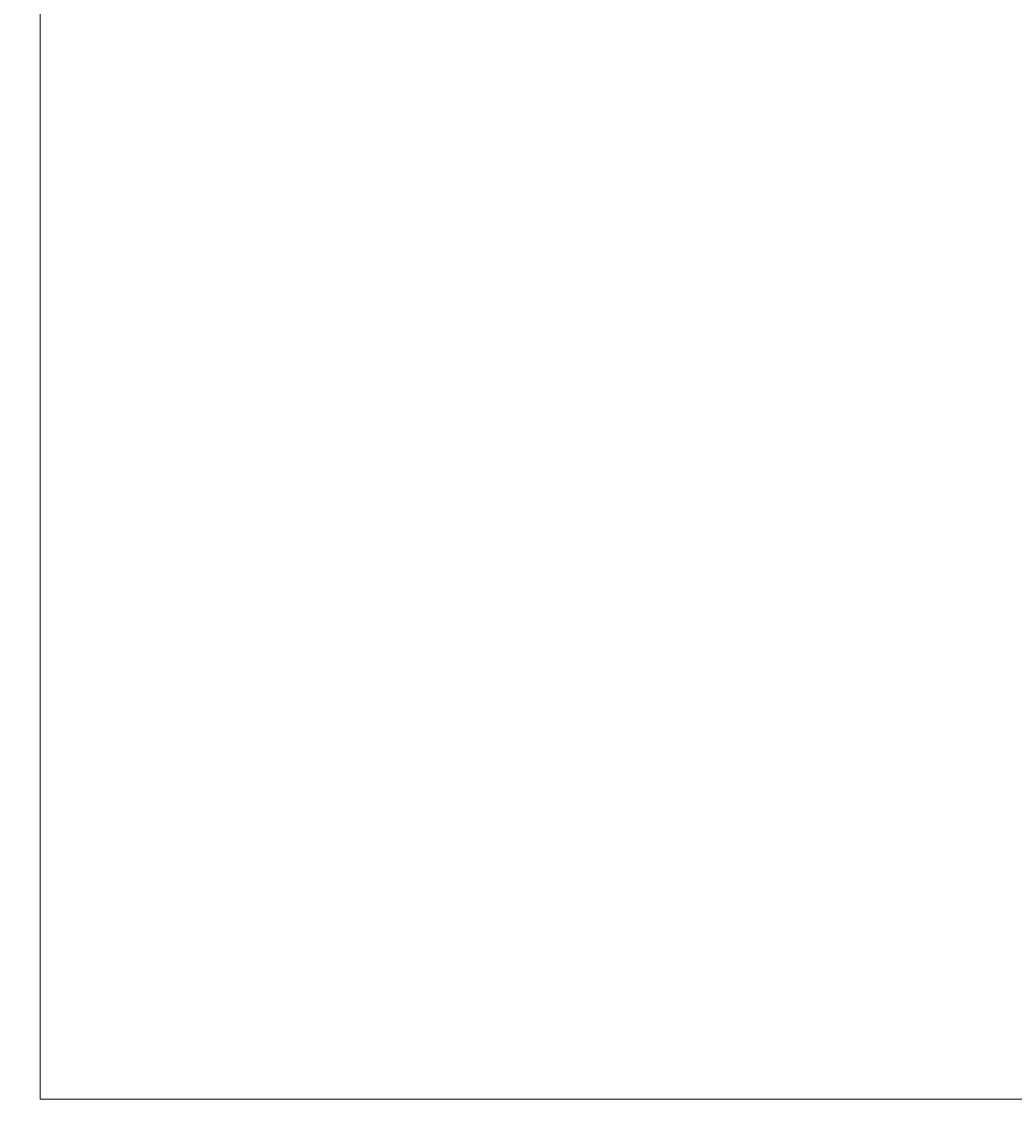
# Model space of a CAD drawing. Units: inches. Extents: x 1885 to 2748, y 783 to 2421.
# Tile 74 of 117: x 2013 to 2038, y 2093 to 2120. Entities that reach past the tile are written whole.
import ezdxf

# ---------------------------------------------------------------- set-up
doc = ezdxf.new("R2010")
doc.units = ezdxf.units.IN
doc.layers.add('A-ANNO-DIMS', color=2, linetype='Continuous', lineweight=18)
doc.layers.add('A-FLOR-CASE', color=9, linetype='Continuous', lineweight=18)
doc.styles.get("Standard").update_dxf_attribs({"font": 'arial.ttf'})
doc.dimstyles.get("Standard").update_dxf_attribs({"dimtxt": 0.18, "dimasz": 0.18, "dimexe": 0.18, "dimexo": 0.0625, "dimgap": 0.09, "dimtad": 0, "dimtih": 1, "dimtoh": 1, "dimdec": 4, "dimzin": 0, "dimdsep": 46, "dimtxsty": 'Standard', "dimcen": 0.09, "dimadec": 0, "dimazin": 0, "dimtfac": 1, "dimtdec": 4, "dimtofl": 0, "dimtmove": 0, "dimatfit": 3, "dimfxl": 1, "dimtolj": 1, "dimtzin": 0, "dimarcsym": 0})

# ---------------------------------------------------------------- blocks, each defined once
blk = doc.blocks.new('*D48')
at = {"layer": 'A-ANNO-DIMS', "color": 0, "lineweight": -2, "transparency": 16777216}
for p, q in [((1980.711, 2348.006), (1902.844, 2348.006)), ((1903.024, 2347.826), (1903.024, 2114.937)), ((1903.024, 1881.686), (1903.024, 2114.574)), ((2016.711, 1881.506), (1902.844, 1881.506))]:
    blk.add_line(p, q, dxfattribs=at)
at = {"layer": 'A-ANNO-DIMS', "color": 0, "transparency": 16777216}
for points in [[(1902.994, 2347.826), (1903.054, 2347.826), (1903.024, 2348.006)], [(1902.994, 1881.686), (1903.054, 1881.686), (1903.024, 1881.506)]]:
    blk.add_solid(points, dxfattribs=at)
at = {"layer": 'Defpoints', "color": 0, "transparency": 16777216}
for p in [(1903.024, 2348.006), (1980.774, 2348.006), (2016.774, 1881.506)]:
    blk.add_point(p, dxfattribs=at)
at = {"layer": 'A-ANNO-DIMS', "color": 0, "transparency": 16777216, "insert": (1903.024, 2114.756), "char_height": 0.18, "attachment_point": 5}
blk.add_mtext('\\A1;466.5', dxfattribs=at)

msp = doc.modelspace()

# ---------------------------------------------------------------- linework, layer by layer
at = {"layer": 'A-FLOR-CASE'}
for p, q in [((2013.676, 2165.006), (2013.676, 2093.221)), ((2013.676, 2093.221), (2117.274, 2093.221))]:
    msp.add_line(p, q, dxfattribs=at)

# ---------------------------------------------------------------- dimensions: what is measured, and where the dimension line sits
at = {"layer": 'A-ANNO-DIMS'}
dim = msp.add_linear_dim(base=(1903.024, 2348.006), p1=(2016.774, 1881.506), p2=(1980.774, 2348.006), angle=90, dimstyle='Standard', override={"dimdec": 1, "dimlfac": 1, "dimrnd": 0, "dimzin": 0, "dimdsep": 46, "dimlunit": 2}, dxfattribs=at)
dim.commit()
dim.dimension.update_dxf_attribs({"geometry": '*D48', "text_midpoint": (1903.024, 2114.756)})

doc.saveas('drawing.dxf')
